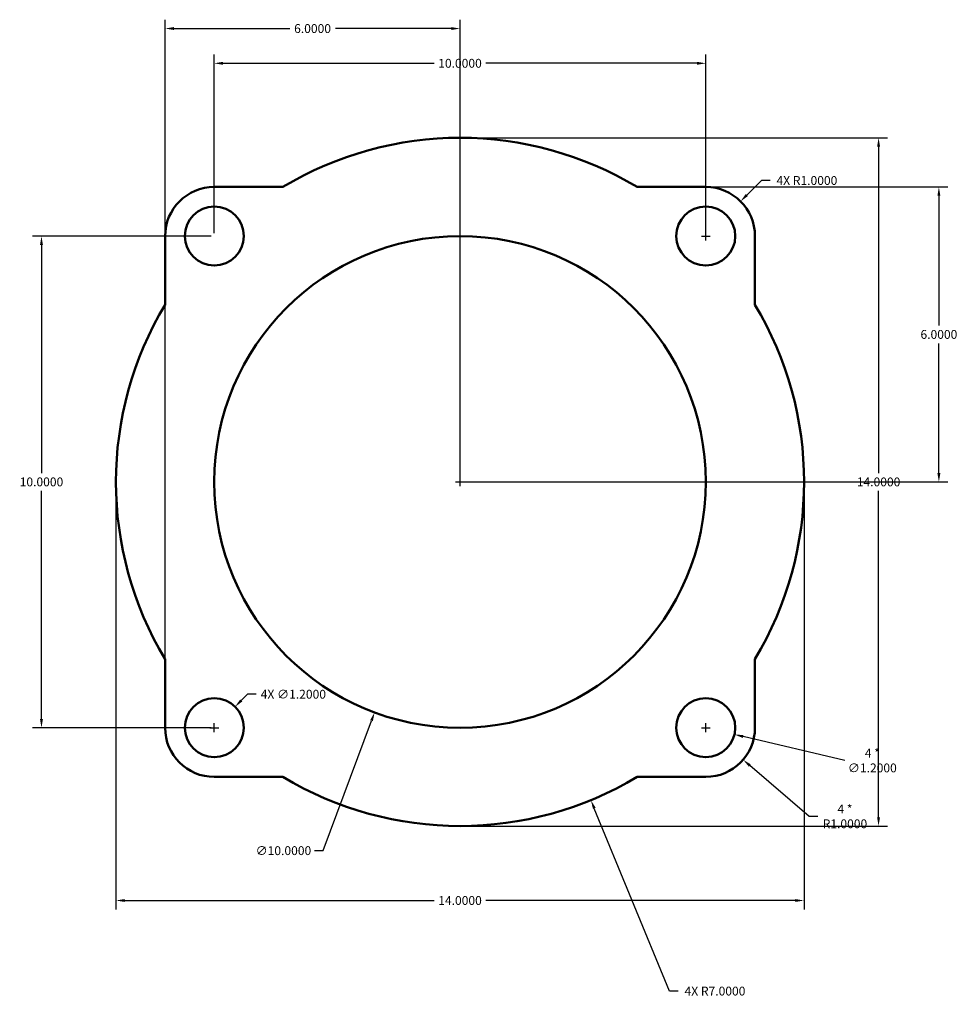
# Model space of a CAD drawing. Units: inches. Extents: x 11.6 to 30.7, y -0.3 to 19.7.
import ezdxf

# ---------------------------------------------------------------- set-up
doc = ezdxf.new("R2010")
doc.units = ezdxf.units.IN
doc.header["$MEASUREMENT"] = 0
doc.layers.add('M-DIMS', color=2, linetype='Continuous', lineweight=25)
doc.layers.add('M-OUTL', color=7, linetype='Continuous', lineweight=50)
doc.styles.get("Standard").update_dxf_attribs({"font": 'arial.ttf'})
doc.dimstyles.get("Standard").update_dxf_attribs({"dimtxt": 0.18, "dimasz": 0.18, "dimexe": 0.18, "dimexo": 0.0625, "dimgap": 0.09, "dimtad": 0, "dimtih": 1, "dimtoh": 1, "dimdec": 4, "dimzin": 0, "dimdsep": 46, "dimtxsty": 'Standard', "dimcen": 0.09, "dimadec": 0, "dimazin": 0, "dimtfac": 1, "dimtdec": 4, "dimtofl": 0, "dimtmove": 0, "dimatfit": 3, "dimfxl": 1, "dimtolj": 1, "dimtzin": 0, "dimarcsym": 0})

# ---------------------------------------------------------------- blocks, each defined once
blk = doc.blocks.new('*D1')
at = {"layer": 'Defpoints', "color": 0, "transparency": 16777216}
for p in [(14.537, 19.546), (20.537, 10.324), (14.537, 5.324)]:
    blk.add_point(p, dxfattribs=at)
at = {"layer": 'M-DIMS', "color": 0, "lineweight": -2, "transparency": 16777216}
for p, q in [((14.537, 5.386), (14.537, 19.726)), ((20.537, 10.386), (20.537, 19.726)), ((14.717, 19.546), (17.073, 19.546)), ((20.357, 19.546), (18.001, 19.546))]:
    blk.add_line(p, q, dxfattribs=at)
at = {"layer": 'M-DIMS', "color": 0, "transparency": 16777216}
for points in [[(14.717, 19.576), (14.717, 19.516), (14.537, 19.546)], [(20.357, 19.576), (20.357, 19.516), (20.537, 19.546)]]:
    blk.add_solid(points, dxfattribs=at)
at = {"layer": 'M-DIMS', "color": 0, "transparency": 16777216, "insert": (17.537, 19.546), "char_height": 0.18, "attachment_point": 5}
blk.add_mtext('\\A1;6.0000', dxfattribs=at)
blk = doc.blocks.new('*D2')
at = {"layer": 'Defpoints', "color": 0, "transparency": 16777216}
for p in [(24.142, 16.324), (20.537, 10.324), (30.279, 10.324)]:
    blk.add_point(p, dxfattribs=at)
at = {"layer": 'M-DIMS', "color": 0, "lineweight": -2, "transparency": 16777216}
for p, q in [((24.205, 16.324), (30.459, 16.324)), ((30.279, 16.144), (30.279, 13.505)), ((30.279, 10.504), (30.279, 13.142)), ((20.599, 10.324), (30.459, 10.324))]:
    blk.add_line(p, q, dxfattribs=at)
at = {"layer": 'M-DIMS', "color": 0, "transparency": 16777216}
for points in [[(30.249, 16.144), (30.309, 16.144), (30.279, 16.324)], [(30.249, 10.504), (30.309, 10.504), (30.279, 10.324)]]:
    blk.add_solid(points, dxfattribs=at)
at = {"layer": 'M-DIMS', "color": 0, "transparency": 16777216, "insert": (30.279, 13.324), "char_height": 0.18, "attachment_point": 5}
blk.add_mtext('\\A1;6.0000', dxfattribs=at)
blk = doc.blocks.new('*D3')
at = {"layer": 'Defpoints', "color": 0, "transparency": 16777216}
for p in [(25.537, 5.324), (26.296, 4.672)]:
    blk.add_point(p, dxfattribs=at)
at = {"layer": 'M-DIMS', "color": 0, "lineweight": -2, "transparency": 16777216}
for p, q in [((25.537, 5.234), (25.537, 5.414)), ((25.447, 5.324), (25.627, 5.324)), ((27.639, 3.519), (26.432, 4.555)), ((27.819, 3.519), (27.639, 3.519))]:
    blk.add_line(p, q, dxfattribs=at)
at = {"layer": 'M-DIMS', "color": 0, "transparency": 16777216}
blk.add_solid([(26.452, 4.578), (26.413, 4.532), (26.296, 4.672)], dxfattribs=at)
at = {"layer": 'M-DIMS', "color": 0, "transparency": 16777216, "insert": (28.368, 3.519), "char_height": 0.18, "attachment_point": 5}
blk.add_mtext('\\A1;4 *\\PR1.0000', dxfattribs=at)
blk = doc.blocks.new('*D4')
at = {"layer": 'Defpoints', "color": 0, "transparency": 16777216}
for p in [(24.953, 5.461), (26.121, 5.186)]:
    blk.add_point(p, dxfattribs=at)
at = {"layer": 'M-DIMS', "color": 0, "lineweight": -2, "transparency": 16777216}
for p, q in [((25.537, 5.234), (25.537, 5.414)), ((25.447, 5.324), (25.627, 5.324)), ((28.364, 4.656), (26.296, 5.144))]:
    blk.add_line(p, q, dxfattribs=at)
at = {"layer": 'M-DIMS', "color": 0, "transparency": 16777216}
blk.add_solid([(26.303, 5.174), (26.289, 5.115), (26.121, 5.186)], dxfattribs=at)
at = {"layer": 'M-DIMS', "color": 0, "transparency": 16777216, "insert": (28.925, 4.656), "char_height": 0.18, "attachment_point": 5}
blk.add_mtext('\\A1;4 *\\P∅1.2000', dxfattribs=at)
blk = doc.blocks.new('MOUNT-HOLE-D1_20IN')
blk.add_circle((0.6, 0.6), 0.6)
blk = doc.blocks.new('*D6')
at = {"layer": 'Defpoints', "color": 0, "transparency": 16777216}
for p in [(25.537, 18.839), (15.537, 15.324), (25.537, 15.324)]:
    blk.add_point(p, dxfattribs=at)
at = {"layer": 'M-DIMS', "color": 0, "lineweight": -2, "transparency": 16777216}
for p, q in [((15.537, 15.386), (15.537, 19.019)), ((15.717, 18.839), (20.012, 18.839)), ((25.357, 18.839), (21.062, 18.839)), ((25.537, 15.386), (25.537, 19.019))]:
    blk.add_line(p, q, dxfattribs=at)
at = {"layer": 'M-DIMS', "color": 0, "transparency": 16777216}
for points in [[(15.717, 18.869), (15.717, 18.809), (15.537, 18.839)], [(25.357, 18.869), (25.357, 18.809), (25.537, 18.839)]]:
    blk.add_solid(points, dxfattribs=at)
at = {"layer": 'M-DIMS', "color": 0, "transparency": 16777216, "insert": (20.537, 18.839), "char_height": 0.18, "attachment_point": 5}
blk.add_mtext('\\A1;10.0000', dxfattribs=at)
blk = doc.blocks.new('*D7')
at = {"layer": 'Defpoints', "color": 0, "transparency": 16777216}
for p in [(12.022, 15.324), (15.537, 15.324), (15.537, 5.324)]:
    blk.add_point(p, dxfattribs=at)
at = {"layer": 'M-DIMS', "color": 0, "lineweight": -2, "transparency": 16777216}
for p, q in [((15.474, 15.324), (11.842, 15.324)), ((12.022, 15.144), (12.022, 10.505)), ((12.022, 5.504), (12.022, 10.142)), ((15.474, 5.324), (11.842, 5.324))]:
    blk.add_line(p, q, dxfattribs=at)
at = {"layer": 'M-DIMS', "color": 0, "transparency": 16777216}
for points in [[(11.992, 15.144), (12.052, 15.144), (12.022, 15.324)], [(11.992, 5.504), (12.052, 5.504), (12.022, 5.324)]]:
    blk.add_solid(points, dxfattribs=at)
at = {"layer": 'M-DIMS', "color": 0, "transparency": 16777216, "insert": (12.022, 10.324), "char_height": 0.18, "attachment_point": 5}
blk.add_mtext('\\A1;10.0000', dxfattribs=at)
blk = doc.blocks.new('*D8')
at = {"layer": 'Defpoints', "color": 0, "transparency": 16777216}
for p in [(13.537, 10.324), (27.537, 10.324), (27.537, 1.809)]:
    blk.add_point(p, dxfattribs=at)
at = {"layer": 'M-DIMS', "color": 0, "lineweight": -2, "transparency": 16777216}
for p, q in [((13.537, 10.261), (13.537, 1.629)), ((27.537, 10.261), (27.537, 1.629)), ((13.717, 1.809), (20.012, 1.809)), ((27.357, 1.809), (21.062, 1.809))]:
    blk.add_line(p, q, dxfattribs=at)
at = {"layer": 'M-DIMS', "color": 0, "transparency": 16777216}
for points in [[(13.717, 1.839), (13.717, 1.779), (13.537, 1.809)], [(27.357, 1.839), (27.357, 1.779), (27.537, 1.809)]]:
    blk.add_solid(points, dxfattribs=at)
at = {"layer": 'M-DIMS', "color": 0, "transparency": 16777216, "insert": (20.537, 1.809), "char_height": 0.18, "attachment_point": 5}
blk.add_mtext('\\A1;14.0000', dxfattribs=at)
blk = doc.blocks.new('*D9')
at = {"layer": 'Defpoints', "color": 0, "transparency": 16777216}
for p in [(20.537, 17.324), (29.052, 17.324), (20.537, 3.324)]:
    blk.add_point(p, dxfattribs=at)
at = {"layer": 'M-DIMS', "color": 0, "lineweight": -2, "transparency": 16777216}
for p, q in [((20.599, 17.324), (29.232, 17.324)), ((29.052, 17.144), (29.052, 10.505)), ((29.052, 3.504), (29.052, 10.142)), ((20.599, 3.324), (29.232, 3.324))]:
    blk.add_line(p, q, dxfattribs=at)
at = {"layer": 'M-DIMS', "color": 0, "transparency": 16777216}
for points in [[(29.022, 17.144), (29.082, 17.144), (29.052, 17.324)], [(29.022, 3.504), (29.082, 3.504), (29.052, 3.324)]]:
    blk.add_solid(points, dxfattribs=at)
at = {"layer": 'M-DIMS', "color": 0, "transparency": 16777216, "insert": (29.052, 10.324), "char_height": 0.18, "attachment_point": 5}
blk.add_mtext('\\A1;14.0000', dxfattribs=at)
blk = doc.blocks.new('*D10')
at = {"layer": 'Defpoints', "color": 0, "transparency": 16777216}
for p in [(22.275, 15.012), (18.798, 5.635)]:
    blk.add_point(p, dxfattribs=at)
at = {"layer": 'M-DIMS', "color": 0, "lineweight": -2, "transparency": 16777216}
for p, q in [((20.447, 10.324), (20.627, 10.324)), ((20.537, 10.234), (20.537, 10.414)), ((17.755, 2.823), (18.736, 5.467)), ((17.575, 2.823), (17.755, 2.823))]:
    blk.add_line(p, q, dxfattribs=at)
at = {"layer": 'M-DIMS', "color": 0, "transparency": 16777216}
blk.add_solid([(18.708, 5.477), (18.764, 5.456), (18.798, 5.635)], dxfattribs=at)
at = {"layer": 'M-DIMS', "color": 0, "transparency": 16777216, "insert": (16.944, 2.823), "char_height": 0.18, "attachment_point": 5}
blk.add_mtext('\\A1;∅10.0000', dxfattribs=at)
blk = doc.blocks.new('*D11')
at = {"layer": 'Defpoints', "color": 0, "transparency": 16777216}
for p in [(20.537, 10.324), (23.2, 3.85)]:
    blk.add_point(p, dxfattribs=at)
at = {"layer": 'M-DIMS', "color": 0, "lineweight": -2, "transparency": 16777216}
for p, q in [((20.447, 10.324), (20.627, 10.324)), ((20.537, 10.234), (20.537, 10.414)), ((24.798, -0.034), (23.269, 3.683)), ((24.978, -0.034), (24.798, -0.034))]:
    blk.add_line(p, q, dxfattribs=at)
at = {"layer": 'M-DIMS', "color": 0, "transparency": 16777216}
blk.add_solid([(23.296, 3.695), (23.241, 3.672), (23.2, 3.85)], dxfattribs=at)
at = {"layer": 'M-DIMS', "color": 0, "transparency": 16777216, "insert": (25.724, -0.034), "char_height": 0.18, "attachment_point": 5}
blk.add_mtext('\\A1;4X R7.0000', dxfattribs=at)
blk = doc.blocks.new('*D12')
at = {"layer": 'Defpoints', "color": 0, "transparency": 16777216}
for p in [(15.959, 5.749), (15.114, 4.898)]:
    blk.add_point(p, dxfattribs=at)
at = {"layer": 'M-DIMS', "color": 0, "lineweight": -2, "transparency": 16777216}
for p, q in [((16.213, 6.005), (16.086, 5.877)), ((16.393, 6.005), (16.213, 6.005)), ((15.537, 5.234), (15.537, 5.414)), ((15.447, 5.324), (15.627, 5.324))]:
    blk.add_line(p, q, dxfattribs=at)
at = {"layer": 'M-DIMS', "color": 0, "transparency": 16777216}
blk.add_solid([(16.065, 5.898), (16.107, 5.856), (15.959, 5.749)], dxfattribs=at)
at = {"layer": 'M-DIMS', "color": 0, "transparency": 16777216, "insert": (17.146, 6.005), "char_height": 0.18, "attachment_point": 5}
blk.add_mtext('\\A1;4X ∅1.2000', dxfattribs=at)
blk = doc.blocks.new('*D13')
at = {"layer": 'Defpoints', "color": 0, "transparency": 16777216}
for p in [(26.244, 16.031), (25.537, 15.324)]:
    blk.add_point(p, dxfattribs=at)
at = {"layer": 'M-DIMS', "color": 0, "lineweight": -2, "transparency": 16777216}
for p, q in [((26.668, 16.455), (26.371, 16.158)), ((26.848, 16.455), (26.668, 16.455)), ((25.447, 15.324), (25.627, 15.324)), ((25.537, 15.234), (25.537, 15.414))]:
    blk.add_line(p, q, dxfattribs=at)
at = {"layer": 'M-DIMS', "color": 0, "transparency": 16777216}
blk.add_solid([(26.35, 16.179), (26.392, 16.137), (26.244, 16.031)], dxfattribs=at)
at = {"layer": 'M-DIMS', "color": 0, "transparency": 16777216, "insert": (27.594, 16.455), "char_height": 0.18, "attachment_point": 5}
blk.add_mtext('\\A1;4X R1.0000', dxfattribs=at)

msp = doc.modelspace()

# ---------------------------------------------------------------- linework, layer by layer
at = {"layer": 'M-OUTL'}
for p, q in [((16.93121, 16.3235), (15.53676, 16.3235)), ((24.14231, 16.3235), (25.53676, 16.3235)), ((14.53676, 15.3235), (14.53676, 13.92906)), ((26.53676, 15.3235), (26.53676, 13.92906)), ((14.53676, 6.71795), (14.53676, 5.3235)), ((26.53676, 6.71795), (26.53676, 5.3235)), ((16.93121, 4.3235), (15.53676, 4.3235)), ((25.53676, 4.3235), (24.14231, 4.3235))]:
    msp.add_line(p, q, dxfattribs=at)
msp.add_circle((20.53676, 10.3235), 5, dxfattribs=at)
for centre, radius, start, end in [((20.53676, 10.3235), 7, 58.997281, 121.002719), ((15.53676, 15.3235), 1, 90, 180), ((25.53676, 15.3235), 1, 0, 90), ((20.53676, 10.3235), 7, 148.997281, 211.002719), ((20.53676, 10.3235), 7, 328.997281, 31.002719), ((15.53676, 5.3235), 1, 180, 270), ((25.53676, 5.3235), 1, 270, 0), ((20.53676, 10.3235), 7, 238.997281, 301.002719)]:
    msp.add_arc(centre, radius, start, end, dxfattribs=at)

# ---------------------------------------------------------------- block references
for p in [(14.937, 14.724), (24.937, 14.724), (14.937, 4.724), (24.937, 4.724)]:
    msp.add_blockref('MOUNT-HOLE-D1_20IN', p, dxfattribs=at)

# ---------------------------------------------------------------- dimensions: what is measured, and where the dimension line sits
at = {"layer": 'M-DIMS'}
for base, p1, p2, override, picture, middle in [((14.53676, 19.546), (20.53676, 10.3235), (14.53676, 5.3235), {"dimclrd": 0, "dimclre": 0, "dimclrt": 0}, '*D1', (17.53676, 19.546)), ((25.53676, 18.8385), (15.53676, 15.3235), (25.53676, 15.3235), {"dimdec": 4, "dimlfac": 1, "dimrnd": 0, "dimzin": 0, "dimdsep": 46, "dimlunit": 2}, '*D6', (20.53676, 18.8385)), ((27.53676, 1.8085), (13.53676, 10.3235), (27.53676, 10.3235), {"dimdec": 4, "dimlfac": 1, "dimrnd": 0, "dimzin": 0, "dimdsep": 46, "dimlunit": 2}, '*D8', (20.53676, 1.8085))]:
    dim = msp.add_linear_dim(base=base, p1=p1, p2=p2, dimstyle='Standard', override=override, dxfattribs=at)
    dim.commit()
    dim.dimension.update_dxf_attribs({"geometry": picture, "text_midpoint": middle})
for base, p1, p2, override, picture, middle in [((29.05176, 17.3235), (20.53676, 3.3235), (20.53676, 17.3235), {"dimdec": 4, "dimlfac": 1, "dimrnd": 0, "dimzin": 0, "dimdsep": 46, "dimlunit": 2}, '*D9', (29.05176, 10.3235)), ((30.27894, 10.3235), (24.14231, 16.3235), (20.53676, 10.3235), {"dimclrd": 0, "dimclre": 0, "dimclrt": 0}, '*D2', (30.27894, 13.3235)), ((12.02176, 15.3235), (15.53676, 5.3235), (15.53676, 15.3235), {"dimdec": 4, "dimlfac": 1, "dimrnd": 0, "dimzin": 0, "dimdsep": 46, "dimlunit": 2}, '*D7', (12.02176, 10.3235))]:
    dim = msp.add_linear_dim(base=base, p1=p1, p2=p2, angle=90, dimstyle='Standard', override=override, dxfattribs=at)
    dim.commit()
    dim.dimension.update_dxf_attribs({"geometry": picture, "text_midpoint": middle})
for center, mpoint, text, override, picture, middle in [((25.53676, 15.3235), (26.24374, 16.03074), '4X <>', {"dimdec": 4, "dimlfac": 1, "dimrnd": 0, "dimzin": 0, "dimdsep": 46, "dimlunit": 2}, '*D13', (27.59439, 16.45508)), ((20.53676, 10.3235), (23.20002, 3.84994), '4X <>', {"dimdec": 4, "dimlfac": 1, "dimrnd": 0, "dimzin": 0, "dimdsep": 46, "dimlunit": 2}, '*D11', (25.72444, -0.0342)), ((25.53676, 5.3235), (26.29556, 4.67218), '4 *\\P<>', {"dimclrd": 0, "dimclre": 0, "dimclrt": 0}, '*D3', (28.36837, 3.51909))]:
    dim = msp.add_radius_dim(center=center, mpoint=mpoint, text=text, dimstyle='Standard', override=override, dxfattribs=at)
    dim.commit()
    dim.dimension.update_dxf_attribs({"geometry": picture, "text_midpoint": middle, "dimtype": 164})
dim = msp.add_diameter_dim_2p(p1=(22.2752, 15.01155), p2=(18.79831, 5.63545), dimstyle='Standard', override={"dimdec": 4, "dimlfac": 1, "dimrnd": 0, "dimzin": 0, "dimdsep": 46, "dimlunit": 2}, dxfattribs=at)
dim.commit()
dim.dimension.update_dxf_attribs({"geometry": '*D10', "text_midpoint": (16.94408, 2.82262), "dimtype": 163})
for p1, p2, text, override, picture, middle in [((15.11412, 4.89762), (15.95939, 5.74939), '4X <>', {"dimdec": 4, "dimlfac": 1, "dimrnd": 0, "dimzin": 0, "dimdsep": 46, "dimlunit": 2}, '*D12', (17.14643, 6.00492)), ((24.95279, 5.46129), (26.12072, 5.18571), '4 *\\P<>', {"dimclrd": 0, "dimclre": 0, "dimclrt": 0}, '*D4', (28.36363, 4.65648))]:
    dim = msp.add_diameter_dim_2p(p1=p1, p2=p2, text=text, dimstyle='Standard', override=override, dxfattribs=at)
    dim.commit()
    dim.dimension.update_dxf_attribs({"geometry": picture, "text_midpoint": middle, "dimtype": 163})

doc.saveas('drawing.dxf')
